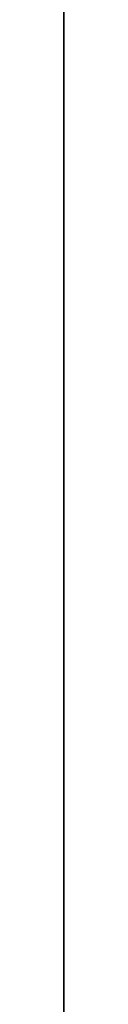
# Model space of a CAD drawing. Units: inches. Extents: x 2083 to 3317, y 1141 to 2115.
# Tile 45 of 256: x 2235.9598 to 2235.9598, y 1478.7355 to 1479.2752. Entities that reach past the tile are written whole.
import ezdxf

# ---------------------------------------------------------------- set-up
doc = ezdxf.new("R2010")
doc.units = ezdxf.units.IN
doc.layers.add('A-ANNO-DIMS', color=2, linetype='Continuous', lineweight=18)
doc.layers.add('A-WALL', color=7, linetype='Continuous', lineweight=35)
doc.layers.add('A-WALL-PATT', color=251, linetype='Continuous', lineweight=13, true_color=0x636466)
doc.styles.get("Standard").update_dxf_attribs({"font": 'arial.ttf'})
doc.dimstyles.new('ISO-25', dxfattribs={"dimtxt": 12, "dimasz": 12, "dimexe": 1.25, "dimexo": 0.625, "dimtad": 1, "dimlunit": 3, "dimtxsty": 'Standard', "dimcen": 2.5, "dimadec": 0, "dimazin": 0, "dimtfac": 1, "dimtmove": 0, "dimatfit": 3, "dimfxl": 1, "dimarcsym": 0})

# ---------------------------------------------------------------- blocks, each defined once
blk = doc.blocks.new('*D30')
at = {"layer": 'A-ANNO-DIMS', "color": 0, "lineweight": -2, "transparency": 16777216}
for p, q in [((2240.01786, 1445.27381), (2240.01786, 1448.04553)), ((2254.32933, 1445.27381), (2254.32933, 1448.04553)), ((2228.01786, 1446.79553), (2216.01786, 1446.79553)), ((2240.01786, 1446.79553), (2254.32933, 1446.79553)), ((2266.32933, 1446.79553), (2413.76487, 1446.79553))]:
    blk.add_line(p, q, dxfattribs=at)
at = {"layer": 'A-ANNO-DIMS', "color": 0, "transparency": 16777216}
for points in [[(2228.01786, 1448.79553), (2228.01786, 1444.79553), (2240.01786, 1446.79553)], [(2266.32933, 1448.79553), (2266.32933, 1444.79553), (2254.32933, 1446.79553)]]:
    blk.add_solid(points, dxfattribs=at)
at = {"layer": 'Defpoints', "color": 0, "transparency": 16777216}
for p in [(2254.32933, 1446.79553), (2240.01786, 1444.64881), (2254.32933, 1444.64881)]:
    blk.add_point(p, dxfattribs=at)
at = {"layer": 'A-ANNO-DIMS', "color": 0, "transparency": 16777216, "insert": (2346.0471, 1453.62517), "char_height": 12, "attachment_point": 5}
blk.add_mtext('WC 1\'-2 1/2" TYP.', dxfattribs=at)
blk = doc.blocks.new('*D31')
at = {"layer": 'A-ANNO-DIMS', "color": 0, "lineweight": -2, "transparency": 16777216}
for p, q in [((2237.87114, 1456.64881), (2237.87114, 1541.91518)), ((2239.39286, 1444.64881), (2236.62114, 1444.64881)), ((2237.87114, 1431.54754), (2237.87114, 1444.64881)), ((2239.39286, 1431.54754), (2236.62114, 1431.54754)), ((2237.87114, 1419.54754), (2237.87114, 1407.54754))]:
    blk.add_line(p, q, dxfattribs=at)
at = {"layer": 'A-ANNO-DIMS', "color": 0, "transparency": 16777216}
for points in [[(2235.87114, 1456.64881), (2239.87114, 1456.64881), (2237.87114, 1444.64881)], [(2235.87114, 1419.54754), (2239.87114, 1419.54754), (2237.87114, 1431.54754)]]:
    blk.add_solid(points, dxfattribs=at)
at = {"layer": 'Defpoints', "color": 0, "transparency": 16777216}
for p in [(2237.87114, 1444.64881), (2240.01786, 1444.64881), (2240.01786, 1431.54754)]:
    blk.add_point(p, dxfattribs=at)
at = {"layer": 'A-ANNO-DIMS', "color": 0, "transparency": 16777216, "insert": (2231.21749, 1505.28199), "char_height": 12, "attachment_point": 5, "rotation": 90}
blk.add_mtext('1\'-1" TYP.', dxfattribs=at)
blk = doc.blocks.new('*D45')
at = {"layer": 'A-ANNO-DIMS', "color": 0, "lineweight": -2, "transparency": 16777216}
for p, q in [((2235.95978, 1478.38636), (2235.95978, 1531.36136)), ((2418.95978, 1478.38636), (2418.95978, 1531.36136)), ((2247.95978, 1530.11136), (2406.95978, 1530.11136))]:
    blk.add_line(p, q, dxfattribs=at)
at = {"layer": 'A-ANNO-DIMS', "color": 0, "transparency": 16777216}
for points in [[(2247.95978, 1532.11136), (2247.95978, 1528.11136), (2235.95978, 1530.11136)], [(2406.95978, 1532.11136), (2406.95978, 1528.11136), (2418.95978, 1530.11136)]]:
    blk.add_solid(points, dxfattribs=at)
at = {"layer": 'Defpoints', "color": 0, "transparency": 16777216}
for p in [(2418.95978, 1530.11136), (2235.95978, 1477.76136), (2418.95978, 1477.76136)]:
    blk.add_point(p, dxfattribs=at)
at = {"layer": 'A-ANNO-DIMS', "color": 0, "transparency": 16777216, "insert": (2327.45978, 1536.86733), "char_height": 12, "attachment_point": 5}
blk.add_mtext('15\'-3"', dxfattribs=at)
blk = doc.blocks.new('*D62')
at = {"layer": 'A-ANNO-DIMS', "color": 0, "lineweight": -2, "transparency": 16777216}
for p, q in [((2235.95978, 1469.38636), (2235.95978, 1522.36136)), ((2379.95978, 1469.38636), (2379.95978, 1522.36136)), ((2247.95978, 1521.11136), (2367.95978, 1521.11136))]:
    blk.add_line(p, q, dxfattribs=at)
at = {"layer": 'A-ANNO-DIMS', "color": 0, "transparency": 16777216}
for points in [[(2247.95978, 1523.11136), (2247.95978, 1519.11136), (2235.95978, 1521.11136)], [(2367.95978, 1523.11136), (2367.95978, 1519.11136), (2379.95978, 1521.11136)]]:
    blk.add_solid(points, dxfattribs=at)
at = {"layer": 'Defpoints', "color": 0, "transparency": 16777216}
for p in [(2379.95978, 1521.11136), (2235.95978, 1468.76136), (2379.95978, 1468.76136)]:
    blk.add_point(p, dxfattribs=at)
at = {"layer": 'A-ANNO-DIMS', "color": 0, "transparency": 16777216, "insert": (2307.95978, 1527.86324), "char_height": 12, "attachment_point": 5}
blk.add_mtext('12\'-0"', dxfattribs=at)

msp = doc.modelspace()

# ---------------------------------------------------------------- hatches: boundary and pattern name
at = {"layer": 'A-WALL-PATT'}
h = msp.add_hatch(color=256, dxfattribs=at)
h.dxf.hatch_style = 1
h.paths.add_polyline_path([(3126.95978, 2020.76136), (2748.95978, 2020.76136), (2604.95978, 2020.76136), (2226.95978, 2020.76136), (2226.95978, 1702.76136), (2466.95978, 1702.76136), (2466.95978, 1582.76136), (2418.95978, 1582.76136), (2418.95978, 1477.76136), (2226.95978, 1477.76136), (2226.95978, 1263.26136), (2544.95978, 1263.26136), (2544.95978, 1411.76136), (2604.95978, 1411.76136), (2685.95978, 1411.76136), (2685.95978, 1420.76136), (2604.95978, 1420.76136), (2604.95978, 1573.76136), (2604.95978, 1702.76136), (2604.95978, 2011.76136), (2748.95978, 2011.76136), (2748.95978, 1702.76136), (2862.95978, 1702.76136), (2862.95978, 1621.76136), (2871.95978, 1621.76136), (2871.95978, 1702.76136), (2883.95978, 1702.76136), (2883.95978, 1706.93946, -0.026459), (2883.95978, 1711.76136), (2757.95978, 1711.76136), (2757.95978, 1807.76136), (2787.95978, 1807.76136), (2787.95978, 1812.26136), (2757.95978, 1812.26136), (2757.95978, 2011.76136), (2877.95978, 2011.76136), (2877.95978, 1812.26136), (2847.95978, 1812.26136), (2847.95978, 1807.76136), (2889.83574, 1807.76136), (2889.83574, 1812.26136), (2882.45978, 1812.26136), (2882.45978, 2011.76136), (3117.95978, 2011.76136), (3117.95978, 1812.26136), (2937.83574, 1812.26136), (2937.83574, 1807.76136), (2995.70978, 1807.76136), (2995.70978, 1796.11767), (3000.20978, 1796.11767), (3000.20978, 1807.76136), (3117.95978, 1807.76136), (3117.95978, 1711.76136), (3000.20978, 1711.76136), (3000.20978, 1760.11767), (2998.5727, 1760.11767, -0.020711), (2995.70978, 1760.11767), (2995.70978, 1711.76136), (2931.95978, 1711.76136), (2931.95978, 1702.76136), (3126.95978, 1702.76136)])
h.paths.add_polyline_path([(2471.45978, 2011.76136), (2471.45978, 1810.01136), (2462.71694, 1810.01136), (2462.71694, 1805.51136), (2505.95978, 1805.51136), (2505.95978, 1810.01136), (2475.95978, 1810.01136), (2475.95978, 2011.76136), (2595.95978, 2011.76136), (2595.95978, 1810.01136), (2565.95978, 1810.01136), (2565.95978, 1805.51136), (2595.95978, 1805.51136), (2595.95978, 1711.76136), (2235.95978, 1711.76136), (2235.95978, 1805.51136), (2353.70978, 1805.51136), (2353.70978, 1796.05416), (2358.20978, 1796.05416), (2358.20978, 1805.51136), (2414.71694, 1805.51136), (2414.71694, 1810.01136), (2235.95978, 1810.01136), (2235.95978, 2011.76136)], flags=16)
h.paths.add_polyline_path([(2270.20473, 1994.61001), (2270.20473, 1970.61001), (2246.20473, 1970.61001), (2246.20473, 1994.61001)], flags=0)
edge = h.paths.add_edge_path(flags=0)
edge.add_ellipse((2332.02739, 1899.79818), major_axis=(-3.04299, 3.04299), ratio=0.1682525, start_angle=-161.33217, end_angle=-156.30711, ccw=False)
edge.add_ellipse((2333.08204, 1898.74353), major_axis=(-1.05465, 1.05465), ratio=0.4535321, start_angle=-123.37102, end_angle=-94.15911)
edge = h.paths.add_edge_path(flags=0)
edge.add_ellipse((2332.02739, 1968.87629), major_axis=(3.04299, 3.04299), ratio=0.1682525, start_angle=18.66783, end_angle=23.69289)
edge.add_spline(control_points=[(2332.9256, 1970.6911), (2332.22677, 1970.3361), (2330.89371, 1969.65891), (2328.41308, 1970.93214), (2327.20393, 1967.74871), (2324.7096, 1969.95559), (2322.53282, 1967.01235), (2320.01285, 1971.29581), (2317.68031, 1968.15784), (2316.04053, 1967.10205), (2315.4269, 1966.8096)], knot_values=[0, 0, 0, 0, 2.267059, 4.324559, 6.685584, 8.878641, 11.121502, 14.300359, 17.755284, 19.732645, 19.732645, 19.732645, 19.732645], degree=3, periodic=0)
edge.add_ellipse((2332.02739, 1968.87629), major_axis=(3.04299, 3.04299), ratio=0.1682525, start_angle=18.66783, end_angle=23.69289, ccw=False)
edge.add_ellipse((2333.08204, 1969.93094), major_axis=(1.05465, 1.05465), ratio=0.4535321, start_angle=56.62898, end_angle=85.84089, ccw=False)
edge = h.paths.add_edge_path(flags=0)
edge.add_spline(control_points=[(2296.42829, 1967.98791), (2293.6278, 1965.33631), (2287.70362, 1959.72709), (2299.74386, 1949.9957), (2294.53259, 1935.66853), (2290.57323, 1920.60351), (2293.39412, 1909.97369), (2296.18541, 1904.96654)], knot_values=[0.099185, 0.099185, 0.099185, 0.099185, 0.345301, 0.619822, 0.982653, 1.386093, 1.810555, 1.810555, 1.810555, 1.810555], degree=3, periodic=0)
edge.add_spline(control_points=[(2296.18541, 1904.96654), (2297.38358, 1902.6193), (2298.00097, 1901.94931), (2298.55297, 1901.46815)], knot_values=[0.006246, 0.006246, 0.006246, 0.006246, 0.055476, 0.055476, 0.055476, 0.055476], degree=3, periodic=0)
edge.add_spline(control_points=[(2298.55297, 1901.46815), (2297.25861, 1900.92322), (2295.22529, 1900.23213), (2293.06023, 1900.61421), (2292.10142, 1900.78841), (2292.08958, 1900.79057)], knot_values=[0.312835, 0.312835, 0.312835, 0.312835, 0.40178, 0.474987, 0.475903, 0.475903, 0.475903, 0.475903], degree=3, periodic=0)
edge.add_arc((2292.79365, 1904.66411), 3.93701, 215.4209, 259.69818, ccw=False)
edge.add_spline(control_points=[(2289.58531, 1902.3823), (2289.47665, 1902.53509), (2289.36848, 1902.68804), (2289.26086, 1902.84117)], knot_values=[0.102872, 0.102872, 0.102872, 0.102872, 0.116896, 0.116896, 0.116896, 0.116896], degree=3, periodic=0)
edge.add_spline(control_points=[(2289.26086, 1902.84117), (2288.6866, 1902.55019), (2287.64005, 1902.0199), (2285.88134, 1901.87395), (2283.85297, 1901.50435), (2281.71999, 1899.71054), (2278.46699, 1899.49294), (2276.15714, 1901.8832), (2272.25895, 1899.80407), (2267.77761, 1901.84318), (2262.24388, 1900.18403), (2257.41493, 1901.78206), (2254.31837, 1900.72612), (2253.17828, 1900.33734)], knot_values=[0, 0, 0, 0, 1.907977, 3.477176, 5.261074, 7.972851, 11.680248, 13.717921, 16.939592, 22.789562, 27.502503, 33.595215, 37.145618, 37.145618, 37.145618, 37.145618], degree=3, periodic=0)
edge.add_line((2253.17828, 1900.33734), (2250.24424, 1902.84117))
edge.add_line((2250.24424, 1902.84117), (2250.24424, 1965.8333))
edge.add_line((2250.24424, 1965.8333), (2253.17828, 1968.33712))
edge.add_spline(control_points=[(2253.17828, 1968.33712), (2254.31837, 1967.94835), (2257.41493, 1966.89241), (2262.24388, 1968.49043), (2267.77761, 1966.83128), (2271.52673, 1968.53722), (2273.87591, 1967.82829), (2274.2067, 1967.72764)], knot_values=[0, 0, 0, 0, 0.09018, 0.244935, 0.364644, 0.513233, 0.537855, 0.537855, 0.537855, 0.537855], degree=3, periodic=0)
edge.add_arc((2274.35289, 1963.79335), 3.93701, 72.05113, 92.12795, ccw=False)
edge.add_arc((2281.29693, 1985.23), 18.5963, 252.051134, 288.565722)
edge.add_arc((2292.31672, 1956.02888), 12.64608, 71.026788, 113.778218, ccw=False)
edge = h.paths.add_edge_path(flags=0)
edge.add_spline(control_points=[(2274.89941, 1951.85619), (2275.06616, 1951.61659), (2275.23269, 1951.37659), (2275.39799, 1951.13585)], knot_values=[1.409916, 1.409916, 1.409916, 1.409916, 1.43159, 1.43159, 1.43159, 1.43159], degree=3, periodic=0)
edge.add_spline(control_points=[(2275.39799, 1951.13585), (2275.79211, 1950.56189), (2276.17923, 1949.98377), (2276.54555, 1949.3971)], knot_values=[1.358238, 1.358238, 1.358238, 1.358238, 1.409916, 1.409916, 1.409916, 1.409916], degree=3, periodic=0)
edge.add_line((2276.54555, 1949.3971), (2277.43729, 1947.86218))
edge.add_spline(control_points=[(2277.43729, 1947.86218), (2276.30383, 1945.67311), (2274.6397, 1942.42688), (2274.63161, 1938.0939), (2272.79912, 1930.85155), (2274.35643, 1943.89705), (2275.94768, 1947.92336), (2276.54555, 1949.3971)], knot_values=[0.005632, 0.005632, 0.005632, 0.005632, 0.186014, 0.266002, 0.357087, 0.59639, 0.739732, 0.739732, 0.739732, 0.739732], degree=3, periodic=0)
edge.add_spline(control_points=[(2276.54555, 1949.3971), (2276.17923, 1949.98377), (2275.79211, 1950.56189), (2275.39799, 1951.13585)], knot_values=[1.358238, 1.358238, 1.358238, 1.358238, 1.409916, 1.409916, 1.409916, 1.409916], degree=3, periodic=0)
edge.add_spline(control_points=[(2275.39799, 1951.13585), (2274.9425, 1950.08045), (2274.20776, 1948.02527), (2273.9346, 1944.85148), (2272.46853, 1937.62749), (2273.46622, 1945.69647), (2274.70062, 1951.05947), (2274.89941, 1951.85619)], knot_values=[0.104364, 0.104364, 0.104364, 0.104364, 0.189636, 0.269624, 0.36071, 0.600013, 0.644622, 0.644622, 0.644622, 0.644622], degree=3, periodic=0)
h.paths.add_polyline_path([(2269.16751, 1963.12757, -0.357527), (2268.17063, 1960.97637, -0.092561), (2268.17063, 1939.43632, -0.357527), (2269.16751, 1937.28512, -0.357527), (2267.01631, 1938.282, -0.164785), (2254.68558, 1938.282, -0.357527), (2252.53438, 1937.28512, -0.357527), (2253.53126, 1939.43632, -0.092561), (2253.53126, 1960.97637, -0.357527), (2252.53438, 1963.12757, -0.357527), (2254.68558, 1962.13069, -0.164785), (2267.01631, 1962.13069, -0.357527)], flags=0)
h.paths.add_polyline_path([(2248.87407, 1967.8018), (2248.87407, 1957.02771), (2249.45778, 1957.02771), (2249.45778, 1911.64676), (2248.87407, 1911.64676), (2248.87407, 1900.87267), (2246.51186, 1900.87267, 0.197327), (2244.14966, 1902.45687), (2244.14966, 1966.21759, 0.197327), (2246.51186, 1967.8018)], flags=0)
h.paths.add_polyline_path([(2269.16751, 1931.38934, -0.357527), (2268.17063, 1929.23814, -0.092561), (2268.17063, 1907.6981, -0.357527), (2269.16751, 1905.54689, -0.357527), (2267.01631, 1906.54377, -0.164785), (2254.68558, 1906.54377, -0.357527), (2252.53438, 1905.54689, -0.357527), (2253.53126, 1907.6981, -0.092561), (2253.53126, 1929.23814, -0.357527), (2252.53438, 1931.38934, -0.357527), (2254.68558, 1930.39246, -0.164785), (2267.01631, 1930.39246, -0.357527)], flags=0)
edge = h.paths.add_edge_path(flags=0)
edge.add_spline(control_points=[(2276.19686, 1906.7237), (2276.16814, 1909.02893), (2276.11405, 1913.37185), (2270.59842, 1924.92498), (2273.90517, 1919.01278), (2275.92171, 1916.26206), (2275.47457, 1912.40215), (2277.25787, 1910.38062), (2276.69604, 1908.22504), (2276.64622, 1906.81302), (2276.61782, 1906.00841)], knot_values=[0, 0, 0, 0, 8.61026, 16.221274, 18.843057, 23.804898, 27.440828, 29.356102, 31.203478, 33.650687, 33.650687, 33.650687, 33.650687], degree=3, periodic=0)
edge.add_spline(control_points=[(2276.61782, 1906.00841), (2276.62331, 1905.62414), (2276.49774, 1904.62866), (2275.44178, 1903.85473), (2274.93731, 1903.08045), (2274.85908, 1902.84117)], knot_values=[0.156488, 0.156488, 0.156488, 0.156488, 0.184398, 0.231376, 0.250598, 0.250598, 0.250598, 0.250598], degree=3, periodic=0)
edge.add_line((2274.85908, 1902.84117), (2276.50598, 1902.84117))
edge.add_spline(control_points=[(2276.50598, 1902.84117), (2276.78831, 1903.08494), (2277.66507, 1904.1252), (2278.24954, 1904.34074), (2277.65387, 1908.52739), (2278.15567, 1906.22781), (2278.10046, 1905.28595), (2278.84667, 1904.06901), (2277.85679, 1903.41495), (2277.87419, 1902.99105), (2277.90356, 1902.84117)], knot_values=[0.059574, 0.059574, 0.059574, 0.059574, 0.080753, 0.103741, 0.16972, 0.176036, 0.207137, 0.240474, 0.262341, 0.27366, 0.27366, 0.27366, 0.27366], degree=3, periodic=0)
edge.add_line((2277.90356, 1902.84117), (2280.02983, 1902.84117))
edge.add_spline(control_points=[(2280.02983, 1902.84117), (2279.88822, 1903.0884), (2279.49926, 1903.98155), (2280.15228, 1905.93935), (2278.10362, 1909.65776), (2279.76239, 1907.18529), (2280.3279, 1904.87486), (2280.48511, 1903.48959), (2281.46327, 1903.24943), (2281.75834, 1902.9365), (2281.83404, 1902.84117)], knot_values=[0.013856, 0.013856, 0.013856, 0.013856, 0.034874, 0.088867, 0.107879, 0.126738, 0.158714, 0.193757, 0.217487, 0.226722, 0.226722, 0.226722, 0.226722], degree=3, periodic=0)
edge.add_spline(control_points=[(2281.83404, 1902.84117), (2281.78753, 1902.8267), (2281.64702, 1902.78299), (2281.39553, 1902.85949), (2281.08808, 1902.98524), (2280.72068, 1903.0609), (2280.33345, 1903.02573), (2280.12477, 1902.89888), (2280.02983, 1902.84117)], knot_values=[0, 0, 0, 0, 0.14413, 0.435517, 0.749276, 1.153046, 1.548371, 1.878348, 1.878348, 1.878348, 1.878348], degree=3, periodic=0)
edge.add_line((2280.02983, 1902.84117), (2277.90356, 1902.84117))
edge.add_spline(control_points=[(2277.90356, 1902.84117), (2277.89286, 1902.79586), (2277.8654, 1902.67964), (2277.60748, 1902.68748), (2277.27405, 1902.8007), (2276.83792, 1902.61977), (2276.58381, 1902.78926), (2276.50598, 1902.84117)], knot_values=[0, 0, 0, 0, 0.127189, 0.326199, 0.628009, 1.24357, 1.515331, 1.515331, 1.515331, 1.515331], degree=3, periodic=0)
edge.add_line((2276.50598, 1902.84117), (2274.85908, 1902.84117))
edge.add_spline(control_points=[(2274.85908, 1902.84117), (2274.81444, 1902.89859), (2274.72513, 1903.01345), (2274.49348, 1903.11897), (2274.24429, 1902.96054), (2273.93712, 1903.18494), (2273.61404, 1902.98314), (2273.40832, 1902.88304), (2273.32225, 1902.84117)], knot_values=[0, 0, 0, 0, 0.21843, 0.436957, 0.687977, 0.990379, 1.398396, 1.69185, 1.69185, 1.69185, 1.69185], degree=3, periodic=0)
edge.add_spline(control_points=[(2273.32225, 1902.84117), (2273.61674, 1903.44569), (2274.274, 1904.53825), (2276.02724, 1904.5737), (2276.20696, 1906.58364), (2276.19686, 1906.7237)], knot_values=[0.012227, 0.012227, 0.012227, 0.012227, 0.059472, 0.106218, 0.134458, 0.134458, 0.134458, 0.134458], degree=3, periodic=0)
h.paths.add_polyline_path([(2270.77605, 1897.78983), (2270.77605, 1873.78983), (2246.77605, 1873.78983), (2246.77605, 1897.78983)], flags=0)
h.paths.add_polyline_path([(2353.70978, 1760.00506), (2353.70978, 1760.05416), (2358.20978, 1760.05416, -0.033729)], flags=0)
h.paths.add_polyline_path([(2321.81912, 1737.52919), (2341.99533, 1737.52919, -0.414214), (2343.20327, 1736.32124), (2343.20327, 1721.0206, -0.414214), (2341.99533, 1719.81265), (2321.81912, 1719.81265, -0.414214), (2320.61117, 1721.0206), (2320.61117, 1736.32124, -0.414214)], flags=0)
h.paths.add_polyline_path([(2324.23501, 1736.32124), (2339.57944, 1736.32124, -0.414214), (2341.99533, 1733.90535), (2341.99533, 1725.44973, -0.414214), (2339.57944, 1723.03384), (2333.68059, 1723.03384), (2333.84532, 1722.04547, -0.870646), (2335.4254, 1721.82589, -0.767327), (2333.92269, 1721.42324), (2331.29102, 1721.42324, -0.767327), (2329.78832, 1721.82589, -0.870646), (2331.3684, 1722.04547), (2331.53313, 1723.03384), (2324.23501, 1723.03384, -0.414214), (2321.81912, 1725.44973), (2321.81912, 1733.90535, -0.414214)], flags=0)
h.paths.add_polyline_path([(2570.48379, 1928.61544), (2589.68379, 1928.61544), (2590.16883, 1928.61544), (2590.16883, 1904.9934), (2570.48379, 1904.9934)], flags=0)
h.paths.add_polyline_path([(2574.44732, 1927.26382, -1), (2572.82884, 1927.26382, -1)], flags=0)
h.paths.add_polyline_path([(2573.08987, 1926.94088), (2573.92503, 1927.77604), (2574.14774, 1927.55333), (2573.31258, 1926.71817)], flags=0)
h.paths.add_polyline_path([(2578.77906, 1919.72962, -1), (2571.59166, 1919.72962, -1)], flags=0)
h.paths.add_polyline_path([(2578.38536, 1919.72962, -1), (2571.98536, 1919.72962, -1)], flags=0)
h.paths.add_polyline_path([(2331.59576, 1729.47622, -1), (2333.61795, 1729.47622, -1)], flags=0)
h.paths.add_polyline_path([(2578.03423, 1927.26382, -1), (2576.41574, 1927.26382, -1)], flags=0)
h.paths.add_polyline_path([(2576.68885, 1927.53109), (2576.91156, 1927.7538), (2577.74673, 1926.91863), (2577.52402, 1926.69592)], flags=0)
h.paths.add_polyline_path([(2578.13906, 1909.85954, -1), (2572.23166, 1909.85954, -1)], flags=0)
h.paths.add_polyline_path([(2577.74536, 1909.85954, -1), (2572.62536, 1909.85954, -1)], flags=0)
h.paths.add_polyline_path([(2583.79772, 1927.26382, -1), (2582.17923, 1927.26382, -1)], flags=0)
h.paths.add_polyline_path([(2582.71865, 1927.7538), (2583.55381, 1926.91863), (2583.3311, 1926.69592), (2582.49594, 1927.53109)], flags=0)
h.paths.add_polyline_path([(2582.49594, 1927.53109), (2582.71865, 1927.7538), (2583.55381, 1926.91863), (2583.3311, 1926.69592)], flags=0)
h.paths.add_polyline_path([(2587.73906, 1920.52962, -1), (2581.83166, 1920.52962, -1)], flags=0)
h.paths.add_polyline_path([(2587.34536, 1920.52962, -1), (2582.22536, 1920.52962, -1)], flags=0)
h.paths.add_polyline_path([(2587.38462, 1927.26382, -1), (2585.76613, 1927.26382, -1)], flags=0)
h.paths.add_polyline_path([(2586.08199, 1926.98025), (2586.91716, 1927.81541), (2587.13987, 1927.5927), (2586.3047, 1926.75754)], flags=0)
h.paths.add_polyline_path([(2588.37906, 1910.65954, -1), (2581.19166, 1910.65954, -1)], flags=0)
h.paths.add_polyline_path([(2587.98536, 1910.65954, -1), (2581.58536, 1910.65954, -1)], flags=0)
h.paths.add_polyline_path([(2417.16773, 1729.4779), (2437.34394, 1729.4779, -0.414214), (2438.55188, 1728.26995), (2438.55188, 1712.96931, -0.414214), (2437.34394, 1711.76136), (2417.16773, 1711.76136, -0.414214), (2415.95978, 1712.96931), (2415.95978, 1728.26995, -0.414214)], flags=0)
h.paths.add_polyline_path([(2419.58362, 1728.26995), (2434.92805, 1728.26995, -0.414214), (2437.34394, 1725.85406), (2437.34394, 1717.39844, -0.414214), (2434.92805, 1714.98255), (2429.0292, 1714.98255), (2429.19393, 1713.99418, -0.870646), (2430.77401, 1713.7746, -0.767327), (2429.2713, 1713.37195), (2426.63963, 1713.37195, -0.767327), (2425.13693, 1713.7746, -0.870646), (2426.71701, 1713.99418), (2426.88174, 1714.98255), (2419.58362, 1714.98255, -0.414214), (2417.16773, 1717.39844), (2417.16773, 1725.85406, -0.414214)], flags=0)
h.paths.add_polyline_path([(2419.58362, 1728.26995), (2434.92805, 1728.26995, -0.414214), (2437.34394, 1725.85406), (2437.34394, 1717.39844, -0.414214), (2434.92805, 1714.98255), (2429.0292, 1714.98255), (2428.35812, 1719.00903), (2427.55282, 1719.00903), (2426.88174, 1714.98255), (2419.58362, 1714.98255, -0.414214), (2417.16773, 1717.39844), (2417.16773, 1725.85406, -0.414214)], flags=0)
h.paths.add_polyline_path([(2426.94437, 1721.42492, -1), (2428.96656, 1721.42492, -1)], flags=0)
h.paths.add_polyline_path([(2475.95978, 1702.76136), (2595.95978, 1702.76136), (2595.95978, 1582.76136), (2475.95978, 1582.76136)], flags=16)
h.paths.add_polyline_path([(2427.95978, 1573.76136), (2595.95978, 1573.76136), (2595.95978, 1468.76136), (2595.95978, 1420.76136), (2384.45978, 1420.76136), (2384.45978, 1468.76136), (2427.95978, 1468.76136)], flags=16)
h.paths.add_polyline_path([(2379.95978, 1468.76136), (2379.95978, 1420.76136), (2235.95978, 1420.76136), (2235.95978, 1468.76136)], flags=16)
h.paths.add_polyline_path([(2317.816, 1466.69577), (2337.9922, 1466.69577, -0.414214), (2339.20015, 1465.48782), (2339.20015, 1450.18718, -0.414214), (2337.9922, 1448.97923), (2317.816, 1448.97923, -0.414214), (2316.60805, 1450.18718), (2316.60805, 1465.48782, -0.414214)], flags=0)
h.paths.add_polyline_path([(2320.23189, 1465.48782), (2335.57631, 1465.48782, -0.414214), (2337.9922, 1463.07193), (2337.9922, 1454.61631, -0.414214), (2335.57631, 1452.20042), (2329.67747, 1452.20042), (2329.84219, 1451.21205, -0.870646), (2331.42228, 1450.99247, -0.767327), (2329.91957, 1450.58983), (2327.2879, 1450.58983, -0.767327), (2325.7852, 1450.99247, -0.870646), (2327.36528, 1451.21205), (2327.53001, 1452.20042), (2320.23189, 1452.20042, -0.414214), (2317.816, 1454.61631), (2317.816, 1463.07193, -0.414214)], flags=0)
h.paths.add_polyline_path([(2320.23189, 1465.48782), (2335.57631, 1465.48782, -0.414214), (2337.9922, 1463.07193), (2337.9922, 1454.61631, -0.414214), (2335.57631, 1452.20042), (2329.67747, 1452.20042), (2329.00638, 1456.22691), (2328.20109, 1456.22691), (2327.53001, 1452.20042), (2320.23189, 1452.20042, -0.414214), (2317.816, 1454.61631), (2317.816, 1463.07193, -0.414214)], flags=0)
h.paths.add_polyline_path([(2327.59264, 1458.6428, -1), (2329.61483, 1458.6428, -1)], flags=0)
h.paths.add_polyline_path([(2244.41174, 1433.34045), (2241.92094, 1433.34045, -0.414214), (2240.01786, 1435.24354), (2240.01786, 1440.95281, -0.414211), (2241.92093, 1442.8559), (2244.41174, 1442.8559, -1.976472)], flags=0)
h.paths.add_polyline_path([(2245.35689, 1434.39754, -0.414214), (2245.35689, 1441.79881, -2.144098)], flags=0)
h.paths.add_polyline_path([(2535.95978, 1416.26136), (2535.95978, 1272.26136), (2235.95978, 1272.26136), (2235.95978, 1416.26136)], flags=16)
h.paths.add_polyline_path([(2260.11956, 1384.29284), (2260.11956, 1362.03865), (2237.86537, 1362.03865), (2237.86537, 1384.29284)], flags=0)
edge = h.paths.add_edge_path(flags=0)
edge.add_line((2318.25185, 1362.0933), (2318.1458, 1362.00097))
edge.add_ellipse((2317.44512, 1360.43104), major_axis=(2.82164, 2.82164), ratio=0.1682525, start_angle=18.66783, end_angle=20.94813, ccw=False)
edge.add_ellipse((2318.42305, 1361.40897), major_axis=(0.97793, 0.97793), ratio=0.4535321, start_angle=56.62898, end_angle=70.2262, ccw=False)
edge = h.paths.add_edge_path(flags=0)
edge.add_line((2319.10737, 1295.57108), (2319.01504, 1295.67713))
edge.add_ellipse((2317.44512, 1296.37781), major_axis=(-2.82164, 2.82164), ratio=0.1682525, start_angle=-161.33217, end_angle=-159.05187, ccw=False)
edge.add_ellipse((2318.42305, 1295.39988), major_axis=(-0.97793, 0.97793), ratio=0.4535321, start_angle=-123.37102, end_angle=-109.7738)
edge = h.paths.add_edge_path(flags=0)
edge.add_spline(control_points=[(2284.21035, 1301.17022), (2284.58069, 1300.44472), (2284.89119, 1299.89202), (2285.15955, 1299.46102)], knot_values=[0.039066, 0.039066, 0.039066, 0.039066, 0.055476, 0.055476, 0.055476, 0.055476], degree=3, periodic=0)
edge.add_line((2285.15955, 1299.46102), (2284.21035, 1301.17022))
edge = h.paths.add_edge_path(flags=0)
edge.add_line((2280.41246, 1297.29801), (2283.36999, 1297.03612))
edge.add_line((2283.36999, 1297.03612), (2286.40569, 1297.92631))
edge.add_spline(control_points=[(2286.40569, 1297.92631), (2285.30549, 1297.46312), (2284.34478, 1297.12915), (2283.36999, 1297.03612)], knot_values=[0.394369, 0.394369, 0.394369, 0.394369, 0.475903, 0.475903, 0.475903, 0.475903], degree=3, periodic=0)
edge.add_spline(control_points=[(2283.36999, 1297.03612), (2283.28139, 1297.02767), (2282.31629, 1296.95734), (2281.3125, 1297.13448), (2280.42344, 1297.29602), (2280.41246, 1297.29801)], knot_values=[0.312835, 0.312835, 0.312835, 0.312835, 0.320246, 0.393453, 0.394369, 0.394369, 0.394369, 0.394369], degree=3, periodic=0)
edge = h.paths.add_edge_path(flags=0)
edge.add_line((2284.43556, 1359.60729), (2280.44629, 1355.32805))
edge.add_line((2280.44629, 1355.32805), (2279.57999, 1351.01775))
edge.add_line((2279.57999, 1351.01775), (2282.41297, 1346.58043))
edge.add_spline(control_points=[(2282.41297, 1346.58043), (2283.15333, 1345.58924), (2284.2529, 1344.0289), (2284.80104, 1342.38717), (2284.93516, 1341.80554)], knot_values=[1.240098, 1.240098, 1.240098, 1.240098, 1.332892, 1.382712, 1.382712, 1.382712, 1.382712], degree=3, periodic=0)
edge.add_spline(control_points=[(2284.93516, 1341.80554), (2285.31911, 1340.1406), (2285.23303, 1338.4092), (2284.90994, 1336.65412)], knot_values=[1.097484, 1.097484, 1.097484, 1.097484, 1.240098, 1.240098, 1.240098, 1.240098], degree=3, periodic=0)
edge.add_spline(control_points=[(2284.90994, 1336.65412), (2284.58685, 1334.89904), (2284.02675, 1333.12027), (2283.46264, 1331.36058)], knot_values=[0.95487, 0.95487, 0.95487, 0.95487, 1.097484, 1.097484, 1.097484, 1.097484], degree=3, periodic=0)
edge.add_line((2283.46264, 1331.36058), (2281.89038, 1326.15336))
edge.add_line((2281.89038, 1326.15336), (2280.75626, 1321.05609))
edge.add_line((2280.75626, 1321.05609), (2280.2992, 1316.00198))
edge.add_line((2280.2992, 1316.00198), (2280.71593, 1310.95007))
edge.add_line((2280.71593, 1310.95007), (2282.02809, 1305.97214))
edge.add_line((2282.02809, 1305.97214), (2284.21035, 1301.17022))
edge.add_spline(control_points=[(2284.21035, 1301.17022), (2283.34073, 1302.73019), (2282.6119, 1304.33649), (2282.02809, 1305.97214)], knot_values=[0.099185, 0.099185, 0.099185, 0.099185, 0.241799, 0.241799, 0.241799, 0.241799], degree=3, periodic=0)
edge.add_spline(control_points=[(2282.02809, 1305.97214), (2281.44428, 1307.60778), (2281.00549, 1309.27276), (2280.71593, 1310.95007)], knot_values=[0.241799, 0.241799, 0.241799, 0.241799, 0.384413, 0.384413, 0.384413, 0.384413], degree=3, periodic=0)
edge.add_spline(control_points=[(2280.71593, 1310.95007), (2280.43324, 1312.58761), (2280.28939, 1314.27696), (2280.29889, 1315.96203), (2280.2992, 1316.00198)], knot_values=[0.384413, 0.384413, 0.384413, 0.384413, 0.523647, 0.527028, 0.527028, 0.527028, 0.527028], degree=3, periodic=0)
edge.add_spline(control_points=[(2280.2992, 1316.00198), (2280.31233, 1317.68696), (2280.47787, 1319.36793), (2280.75626, 1321.05609)], knot_values=[0.527028, 0.527028, 0.527028, 0.527028, 0.669642, 0.669642, 0.669642, 0.669642], degree=3, periodic=0)
edge.add_spline(control_points=[(2280.75626, 1321.05609), (2281.03465, 1322.74425), (2281.42588, 1324.43961), (2281.89038, 1326.15336)], knot_values=[0.669642, 0.669642, 0.669642, 0.669642, 0.812256, 0.812256, 0.812256, 0.812256], degree=3, periodic=0)
edge.add_spline(control_points=[(2281.89038, 1326.15336), (2282.26438, 1327.53325), (2282.78787, 1329.26181), (2283.35275, 1331.01778), (2283.46264, 1331.36058)], knot_values=[0.812256, 0.812256, 0.812256, 0.812256, 0.927087, 0.95487, 0.95487, 0.95487, 0.95487], degree=3, periodic=0)
edge.add_line((2283.46264, 1331.36058), (2284.90994, 1336.65412))
edge.add_line((2284.90994, 1336.65412), (2284.93516, 1341.80554))
edge.add_line((2284.93516, 1341.80554), (2282.41297, 1346.58043))
edge.add_spline(control_points=[(2282.41297, 1346.58043), (2281.27513, 1348.10379), (2280.07845, 1349.57032), (2279.57999, 1351.01775)], knot_values=[1.382712, 1.382712, 1.382712, 1.382712, 1.525326, 1.525326, 1.525326, 1.525326], degree=3, periodic=0)
edge.add_spline(control_points=[(2279.57999, 1351.01775), (2279.44328, 1351.41472), (2279.13631, 1352.85692), (2279.73519, 1354.29039), (2280.44629, 1355.32805)], knot_values=[1.525326, 1.525326, 1.525326, 1.525326, 1.564439, 1.667941, 1.667941, 1.667941, 1.667941], degree=3, periodic=0)
edge.add_spline(control_points=[(2280.44629, 1355.32805), (2281.42611, 1356.75784), (2282.93084, 1358.18256), (2284.43556, 1359.60729)], knot_values=[1.667941, 1.667941, 1.667941, 1.667941, 1.810555, 1.810555, 1.810555, 1.810555], degree=3, periodic=0)
edge.add_arc((2280.62307, 1348.51818), 11.72618, 71.026788, 113.778218)
edge.add_arc((2270.40489, 1375.59516), 17.24357, 252.051134, 288.565722, ccw=False)
edge.add_arc((2263.96597, 1355.71785), 3.65062, 72.05113, 92.12795)
edge.add_arc((2263.96597, 1355.71785), 3.65062, 92.12795, 177.98513)
edge.add_spline(control_points=[(2260.3176, 1355.8462), (2260.26042, 1354.22067), (2260.55128, 1350.18655), (2262.99934, 1346.76625), (2264.47274, 1344.64902)], knot_values=[1.43159, 1.43159, 1.43159, 1.43159, 1.564144, 1.770695, 1.770695, 1.770695, 1.770695], degree=3, periodic=0)
edge.add_line((2264.47274, 1344.64902), (2264.93559, 1343.98253))
edge.add_spline(control_points=[(2263.80104, 1340.24811), (2263.84324, 1340.51409), (2264.06724, 1341.75647), (2264.51269, 1343.00245), (2264.93505, 1343.98108)], knot_values=[0.53657, 0.53657, 0.53657, 0.53657, 0.559349, 0.644622, 0.644622, 0.644622, 0.644622], degree=3, periodic=0)
edge.add_spline(control_points=[(2264.93505, 1343.98108), (2265.11777, 1343.71497), (2265.29888, 1343.44791), (2265.47676, 1343.17936)], knot_values=[1.384077, 1.384077, 1.384077, 1.384077, 1.409916, 1.409916, 1.409916, 1.409916], degree=3, periodic=0)
edge.add_spline(control_points=[(2265.47676, 1343.17936), (2265.65464, 1342.91082), (2265.8293, 1342.64081), (2265.99913, 1342.36881)], knot_values=[1.358238, 1.358238, 1.358238, 1.358238, 1.384077, 1.384077, 1.384077, 1.384077], degree=3, periodic=0)
edge.add_line((2265.99913, 1342.36881), (2266.82601, 1340.94555))
edge.add_spline(control_points=[(2266.82601, 1340.94555), (2268.8944, 1337.08969), (2271.39817, 1325.843), (2270.51616, 1310.56856), (2275.91938, 1301.86061), (2277.78951, 1299.19945)], knot_values=[0.116896, 0.116896, 0.116896, 0.116896, 0.472987, 1.050969, 1.313793, 1.313793, 1.313793, 1.313793], degree=3, periodic=0)
edge.add_spline(control_points=[(2277.78951, 1299.19945), (2277.83941, 1299.12845), (2277.88943, 1299.0575), (2277.93957, 1298.98658)], knot_values=[0.109884, 0.109884, 0.109884, 0.109884, 0.116896, 0.116896, 0.116896, 0.116896], degree=3, periodic=0)
edge.add_line((2277.93957, 1298.98658), (2277.78885, 1299.19911))
edge.add_spline(control_points=[(2277.78885, 1299.19911), (2277.25658, 1298.92941), (2276.28635, 1298.4379), (2275.03935, 1298.33442), (2274.38333, 1298.2389), (2274.21525, 1298.20934)], knot_values=[33.12187, 33.12187, 33.12187, 33.12187, 35.029056, 36.598255, 37.144827, 37.144827, 37.144827, 37.144827], degree=3, periodic=0)
edge.add_line((2274.21525, 1298.20934), (2273.07315, 1297.89296))
edge.add_spline(control_points=[(2273.07315, 1297.89296), (2272.32294, 1297.57978), (2271.03915, 1296.51051), (2269.24839, 1296.22606), (2268.4231, 1296.37465)], knot_values=[26.532584, 26.532584, 26.532584, 26.532584, 29.198919, 31.839101, 31.839101, 31.839101, 31.839101], degree=3, periodic=0)
edge.add_line((2268.4231, 1296.37465), (2263.8785, 1297.45753))
edge.add_spline(control_points=[(2263.8785, 1297.45753), (2263.55608, 1297.35943), (2261.86031, 1296.83869), (2260.23878, 1297.28241), (2258.93345, 1297.51646)], knot_values=[15.919551, 15.919551, 15.919551, 15.919551, 16.939592, 21.226067, 21.226067, 21.226067, 21.226067], degree=3, periodic=0)
edge.add_line((2258.93345, 1297.51646), (2254.05523, 1297.32901))
edge.add_spline(control_points=[(2254.05523, 1297.32901), (2253.75553, 1297.29582), (2252.11368, 1297.16517), (2250.46187, 1297.54422), (2249.12969, 1297.66788)], knot_values=[5.306517, 5.306517, 5.306517, 5.306517, 6.276435, 10.613034, 10.613034, 10.613034, 10.613034], degree=3, periodic=0)
edge.add_line((2249.12969, 1297.66788), (2244.33165, 1296.87776))
edge.add_line((2244.33165, 1296.87776), (2241.61103, 1299.19945))
edge.add_line((2241.61103, 1299.19945), (2241.61103, 1357.6094))
edge.add_line((2241.61103, 1357.6094), (2244.33165, 1359.9311))
edge.add_line((2244.33165, 1359.9311), (2252.72882, 1359.54269))
edge.add_spline(control_points=[(2252.72882, 1359.54269), (2252.87094, 1359.54644), (2253.30574, 1359.54817), (2253.73984, 1359.51427), (2254.03174, 1359.48243)], knot_values=[0.233291, 0.233291, 0.233291, 0.233291, 0.244935, 0.268927, 0.268927, 0.268927, 0.268927], degree=3, periodic=0)
edge.add_line((2254.03174, 1359.48243), (2259.58719, 1359.41639))
edge.add_spline(control_points=[(2259.58719, 1359.41639), (2260.67707, 1359.6285), (2262.0732, 1359.897), (2263.52369, 1359.45928), (2263.83042, 1359.36595)], knot_values=[0.422516, 0.422516, 0.422516, 0.422516, 0.513233, 0.537855, 0.537855, 0.537855, 0.537855], degree=3, periodic=0)
edge.add_arc((2263.96597, 1355.71785), 3.65062, 72.05113, 92.12795, ccw=False)
edge.add_arc((2270.40489, 1375.59516), 17.24357, 252.051134, 288.565722)
edge.add_arc((2280.62307, 1348.51818), 11.72618, 71.026788, 113.778218, ccw=False)
h.paths.add_polyline_path([(2240.34053, 1359.43471), (2240.34053, 1349.44435), (2240.88178, 1349.44435), (2240.88178, 1307.3645), (2240.34053, 1307.3645), (2240.34053, 1297.37414), (2238.15016, 1297.37414, 0.197327), (2235.95978, 1298.84311), (2235.95978, 1357.96575, 0.197327), (2238.15016, 1359.43471)], flags=0)
h.paths.add_polyline_path([(2259.15779, 1355.1005, -0.357527), (2258.23342, 1353.10578, -0.092561), (2258.23342, 1333.1326, -0.357527), (2259.15779, 1331.13788, -0.357527), (2257.16307, 1332.06225, -0.164785), (2245.7293, 1332.06225, -0.357527), (2243.73458, 1331.13788, -0.357527), (2244.65895, 1333.1326, -0.092561), (2244.65895, 1353.10578, -0.357527), (2243.73458, 1355.1005, -0.357527), (2245.7293, 1354.17613, -0.164785), (2257.16307, 1354.17613, -0.357527)], flags=0)
edge = h.paths.add_edge_path(flags=0)
edge.add_line((2265.99913, 1342.36881), (2266.82601, 1340.94555))
edge.add_line((2266.82601, 1340.94555), (2265.30756, 1337.81407))
edge.add_line((2265.30756, 1337.81407), (2264.35823, 1334.65294))
edge.add_line((2264.35823, 1334.65294), (2264.26201, 1333.7997))
edge.add_spline(control_points=[(2264.26201, 1333.7997), (2264.20836, 1333.18705), (2264.16206, 1332.36553), (2264.00714, 1331.41393), (2263.96905, 1331.20183)], knot_values=[0.464444, 0.464444, 0.464444, 0.464444, 0.516691, 0.531608, 0.531608, 0.531608, 0.531608], degree=3, periodic=0)
edge.add_spline(control_points=[(2263.96905, 1331.20183), (2263.77453, 1330.11887), (2263.42437, 1328.79084), (2263.25742, 1328.53065), (2263.23403, 1328.51461)], knot_values=[0.372682, 0.372682, 0.372682, 0.372682, 0.44885, 0.464444, 0.464444, 0.464444, 0.464444], degree=3, periodic=0)
edge.add_spline(control_points=[(2263.23403, 1328.51461), (2263.09638, 1328.42023), (2263.13117, 1329.30148), (2263.27495, 1330.61575)], knot_values=[0.280919, 0.280919, 0.280919, 0.280919, 0.372682, 0.372682, 0.372682, 0.372682], degree=3, periodic=0)
edge.add_spline(control_points=[(2263.27495, 1330.61575), (2263.41874, 1331.93002), (2263.67152, 1333.67732), (2263.96985, 1335.31503)], knot_values=[0.189157, 0.189157, 0.189157, 0.189157, 0.280919, 0.280919, 0.280919, 0.280919], degree=3, periodic=0)
edge.add_spline(control_points=[(2263.96985, 1335.31503), (2264.1005, 1336.03219), (2264.41878, 1337.62191), (2264.75485, 1338.86443), (2264.94742, 1339.49112)], knot_values=[0.097394, 0.097394, 0.097394, 0.097394, 0.137578, 0.189157, 0.189157, 0.189157, 0.189157], degree=3, periodic=0)
edge.add_spline(control_points=[(2264.94742, 1339.49112), (2265.29002, 1340.60605), (2265.64424, 1341.494), (2265.99913, 1342.36881)], knot_values=[0.005632, 0.005632, 0.005632, 0.005632, 0.097394, 0.097394, 0.097394, 0.097394], degree=3, periodic=0)
h.paths.add_polyline_path([(2259.15779, 1325.67097, -0.357527), (2258.23342, 1323.67625, -0.092561), (2258.23342, 1303.70307, -0.357527), (2259.15779, 1301.70835, -0.357527), (2257.16307, 1302.63272, -0.164785), (2245.7293, 1302.63272, -0.357527), (2243.73458, 1301.70835, -0.357527), (2244.65895, 1303.70307, -0.092561), (2244.65895, 1323.67625, -0.357527), (2243.73458, 1325.67097, -0.357527), (2245.7293, 1324.74661, -0.164785), (2257.16307, 1324.74661, -0.357527)], flags=0)
edge = h.paths.add_edge_path(flags=0)
edge.add_spline(control_points=[(2261.70894, 1317.31142), (2261.67948, 1317.41758), (2261.76186, 1317.38853), (2262.49074, 1316.08987), (2262.96218, 1315.3009)], knot_values=[14.955861, 14.955861, 14.955861, 14.955861, 16.221274, 18.694826, 18.694826, 18.694826, 18.694826], degree=3, periodic=0)
edge.add_spline(control_points=[(2262.96218, 1315.3009), (2262.99044, 1315.25362), (2263.7021, 1314.06738), (2264.34898, 1313.12715), (2264.73005, 1312.16415)], knot_values=[18.694826, 18.694826, 18.694826, 18.694826, 18.843057, 22.433791, 22.433791, 22.433791, 22.433791], degree=3, periodic=0)
edge.add_spline(control_points=[(2264.73005, 1312.16415), (2264.87556, 1311.79644), (2265.17687, 1310.76981), (2265.14307, 1309.55926), (2265.24774, 1308.82419)], knot_values=[22.433791, 22.433791, 22.433791, 22.433791, 23.804898, 26.172756, 26.172756, 26.172756, 26.172756], degree=3, periodic=0)
edge.add_line((2265.24774, 1308.82419), (2265.85077, 1307.17189))
edge.add_spline(control_points=[(2265.85077, 1307.17189), (2266.06502, 1306.82168), (2266.38439, 1306.33225), (2266.4244, 1305.78055), (2266.42037, 1305.61122)], knot_values=[28.062562, 28.062562, 28.062562, 28.062562, 29.356102, 29.911721, 29.911721, 29.911721, 29.911721], degree=3, periodic=0)
edge.add_spline(control_points=[(2266.42037, 1305.61122), (2266.41612, 1305.43259), (2266.394, 1305.25), (2266.36478, 1305.06586)], knot_values=[29.911721, 29.911721, 29.911721, 29.911721, 30.497837, 30.497837, 30.497837, 30.497837], degree=3, periodic=0)
edge.add_line((2266.36478, 1305.06586), (2266.06615, 1302.1363))
edge.add_spline(control_points=[(2266.06615, 1302.1363), (2266.07124, 1301.77998), (2265.99808, 1301.19998), (2265.66327, 1300.75896), (2265.50891, 1300.58588)], knot_values=[0.156488, 0.156488, 0.156488, 0.156488, 0.184398, 0.203543, 0.203543, 0.203543, 0.203543], degree=3, periodic=0)
edge.add_line((2265.50891, 1300.58588), (2264.43534, 1299.19945))
edge.add_line((2264.43534, 1299.19945), (2265.96244, 1299.19945))
edge.add_line((2265.96244, 1299.19945), (2267.33599, 1301.17528))
edge.add_line((2267.33599, 1301.17528), (2267.31167, 1301.98624))
edge.add_spline(control_points=[(2267.31167, 1301.98624), (2267.26111, 1302.8624), (2267.16021, 1303.73713), (2267.27149, 1303.3259)], knot_values=[0.126229, 0.126229, 0.126229, 0.126229, 0.166617, 0.166617, 0.166617, 0.166617], degree=3, periodic=0)
edge.add_spline(control_points=[(2267.27149, 1303.3259), (2267.28003, 1303.2943), (2267.30979, 1303.17537), (2267.37345, 1302.88361), (2267.40612, 1302.68283), (2267.41793, 1302.60103)], knot_values=[0.166617, 0.166617, 0.166617, 0.166617, 0.16972, 0.176036, 0.180765, 0.180765, 0.180765, 0.180765], degree=3, periodic=0)
edge.add_spline(control_points=[(2267.74389, 1300.9875), (2267.68758, 1301.15094), (2267.48052, 1301.65666), (2267.48375, 1302.14479), (2267.41793, 1302.60103)], knot_values=[0.180765, 0.180765, 0.180765, 0.180765, 0.193767, 0.220139, 0.220139, 0.220139, 0.220139], degree=3, periodic=0)
edge.add_line((2267.41793, 1302.60103), (2267.74389, 1300.9875))
edge.add_spline(control_points=[(2267.74389, 1300.9875), (2267.83196, 1300.73188), (2267.93202, 1300.3099), (2267.55484, 1299.97452), (2267.42937, 1299.82921)], knot_values=[0.220139, 0.220139, 0.220139, 0.220139, 0.240474, 0.25489, 0.25489, 0.25489, 0.25489], degree=3, periodic=0)
edge.add_line((2267.42937, 1299.82921), (2267.25836, 1299.19945))
edge.add_line((2267.25836, 1299.19945), (2269.22996, 1299.19945))
edge.add_spline(control_points=[(2269.22996, 1299.19945), (2269.09865, 1299.42869), (2268.84277, 1300.01625), (2269.01157, 1300.91592), (2268.9468, 1301.66074)], knot_values=[0.013856, 0.013856, 0.013856, 0.013856, 0.034874, 0.067073, 0.067073, 0.067073, 0.067073], degree=3, periodic=0)
edge.add_line((2268.9468, 1301.66074), (2268.43158, 1303.60311))
edge.add_spline(control_points=[(2268.43158, 1303.60311), (2268.1756, 1304.19237), (2267.59621, 1305.2513), (2268.0407, 1304.62321), (2268.25139, 1304.28242)], knot_values=[0.090155, 0.090155, 0.090155, 0.090155, 0.107879, 0.120289, 0.120289, 0.120289, 0.120289], degree=3, periodic=0)
edge.add_spline(control_points=[(2268.25139, 1304.28242), (2268.36088, 1304.10533), (2269.05775, 1302.91798), (2269.38269, 1301.59042), (2269.52141, 1300.77593), (2269.57522, 1300.55578)], knot_values=[0.120289, 0.120289, 0.120289, 0.120289, 0.126738, 0.158714, 0.173506, 0.173506, 0.173506, 0.173506], degree=3, periodic=0)
edge.add_line((2269.57522, 1300.55578), (2270.6858, 1299.42126))
edge.add_spline(control_points=[(2270.6858, 1299.42126), (2270.76722, 1299.35725), (2270.83785, 1299.2814), (2270.90292, 1299.19945)], knot_values=[0.21816, 0.21816, 0.21816, 0.21816, 0.226722, 0.226722, 0.226722, 0.226722], degree=3, periodic=0)
edge.add_line((2270.9372, 1299.19291), (2270.90292, 1299.19945))
edge.add_spline(control_points=[(2270.90292, 1299.19945), (2270.85981, 1299.18603), (2270.72951, 1299.1455), (2270.49631, 1299.21644), (2270.27166, 1299.30832), (2270.12102, 1299.34796), (2270.06334, 1299.35956)], knot_values=[0.939174, 0.939174, 0.939174, 0.939174, 1.083304, 1.374691, 1.68845, 1.878348, 1.878348, 1.878348, 1.878348], degree=3, periodic=0)
edge.add_line((2270.06334, 1299.35956), (2269.22996, 1299.19945))
edge.add_line((2269.22996, 1299.19945), (2267.25836, 1299.19945))
edge.add_spline(control_points=[(2267.25836, 1299.19945), (2267.24843, 1299.15743), (2267.22297, 1299.04967), (2266.98382, 1299.05694), (2266.80921, 1299.11623), (2266.6769, 1299.10909), (2266.63653, 1299.10481)], knot_values=[0.757665, 0.757665, 0.757665, 0.757665, 0.884854, 1.083864, 1.385675, 1.515331, 1.515331, 1.515331, 1.515331], degree=3, periodic=0)
edge.add_spline(control_points=[(2266.63653, 1299.10481), (2266.48522, 1299.08879), (2266.23581, 1299.01712), (2266.03461, 1299.15132), (2265.96244, 1299.19945)], knot_values=[0, 0, 0, 0, 0.485905, 0.757665, 0.757665, 0.757665, 0.757665], degree=3, periodic=0)
edge.add_line((2265.96244, 1299.19945), (2264.43534, 1299.19945))
edge.add_line((2264.43534, 1299.19945), (2263.85844, 1299.36712))
edge.add_spline(control_points=[(2263.85844, 1299.36712), (2263.81894, 1299.37091), (2263.77953, 1299.38572), (2263.74013, 1299.4015)], knot_values=[0.845925, 0.845925, 0.845925, 0.845925, 0.978627, 0.978627, 0.978627, 0.978627], degree=3, periodic=0)
edge.add_line((2263.72179, 1299.39643), (2263.01031, 1299.19945))
edge.add_spline(control_points=[(2263.01031, 1299.19945), (2263.24579, 1299.68286), (2263.50603, 1300.12811), (2263.87349, 1300.40803)], knot_values=[0.012227, 0.012227, 0.012227, 0.012227, 0.052971, 0.052971, 0.052971, 0.052971], degree=3, periodic=0)
edge.add_spline(control_points=[(2263.87349, 1300.40803), (2263.93213, 1300.4527), (2264.08424, 1300.55298), (2264.25519, 1300.62422), (2264.35969, 1300.66475)], knot_values=[0.052971, 0.052971, 0.052971, 0.052971, 0.059472, 0.069086, 0.069086, 0.069086, 0.069086], degree=3, periodic=0)
edge.add_line((2264.35969, 1300.66475), (2265.1419, 1301.07777))
edge.add_line((2265.1419, 1301.07777), (2265.67581, 1302.79956))
edge.add_line((2265.67581, 1302.79956), (2265.5407, 1305.70407))
edge.add_line((2265.5407, 1305.70407), (2264.80307, 1309.32772))
edge.add_line((2264.80307, 1309.32772), (2263.04053, 1314.09179))
edge.add_spline(control_points=[(2263.04053, 1314.09179), (2262.38357, 1315.67144), (2261.79597, 1316.99775), (2261.70894, 1317.31142)], knot_values=[11.216896, 11.216896, 11.216896, 11.216896, 14.955861, 14.955861, 14.955861, 14.955861], degree=3, periodic=0)
h.paths.add_polyline_path([(2871.95978, 1416.26136), (2895.91005, 1416.26136), (2895.91005, 1420.76136), (2871.95978, 1420.76136), (2871.95978, 1501.76136), (2862.95978, 1501.76136), (2862.95978, 1420.76136), (2805.95978, 1420.76136), (2805.95978, 1411.76136), (2862.95978, 1411.76136), (2862.95978, 1263.26136), (3126.95978, 1263.26136), (3126.95978, 1411.76136), (3126.95978, 1486.76136), (2943.95978, 1486.76136), (2943.95978, 1477.76136), (2967.86031, 1477.76136), (2967.86031, 1420.76136), (2943.91005, 1420.76136), (2943.91005, 1416.26136), (3117.95978, 1416.26136), (3117.95978, 1420.76136), (2972.36031, 1420.76136), (2972.36031, 1477.76136), (3117.95978, 1477.76136), (3117.95978, 1420.76136), (3117.95978, 1272.26136), (2871.95978, 1272.26136)], flags=0)
h.paths.add_polyline_path([(2457.12563, 1485.94251), (2527.60265, 1485.94251), (2527.60265, 1537.6357), (2457.12563, 1537.6357)], flags=8)
h.paths.add_polyline_path([(2481.00506, 1609.9818), (2590.76582, 1609.9818), (2590.76582, 1682.00336), (2481.00506, 1682.00336)], flags=8)
h.paths.add_polyline_path([(2483.08502, 1729.12678), (2553.56205, 1729.12678), (2553.56205, 1780.81998), (2483.08502, 1780.81998)], flags=8)

# ---------------------------------------------------------------- linework, layer by layer
at = {"layer": 'A-WALL'}
msp.add_line((2235.95978, 1702.76136), (2235.95978, 1477.76136), dxfattribs=at)
msp.add_line((2235.95978, 1702.76136), (2235.95978, 1477.76136), dxfattribs=at)

# ---------------------------------------------------------------- dimensions: what is measured, and where the dimension line sits
at = {"layer": 'A-ANNO-DIMS'}
for base, p1, p2, picture, middle in [((2418.95978, 1530.11136), (2235.95978, 1477.76136), (2418.95978, 1477.76136), '*D45', (2327.45978, 1536.86733)), ((2379.95978, 1521.11136), (2235.95978, 1468.76136), (2379.95978, 1468.76136), '*D62', (2307.95978, 1527.86324))]:
    dim = msp.add_linear_dim(base=base, p1=p1, p2=p2, dimstyle='ISO-25', override={"dimdec": 1, "dimlfac": 1, "dimrnd": 0, "dimzin": 1, "dimdsep": 46, "dimlunit": 4, "dimfrac": 2}, dxfattribs=at)
    dim.commit()
    dim.dimension.update_dxf_attribs({"geometry": picture, "text_midpoint": middle})
dim = msp.add_linear_dim(base=(2237.87114, 1444.64881), p1=(2240.01786, 1431.54754), p2=(2240.01786, 1444.64881), angle=90, text='<> TYP.', dimstyle='ISO-25', override={"dimdec": 1, "dimlfac": 1, "dimrnd": 0, "dimzin": 1, "dimdsep": 46, "dimlunit": 4, "dimfrac": 2}, dxfattribs=at)
dim.commit()
dim.dimension.update_dxf_attribs({"geometry": '*D31', "text_midpoint": (2231.21749, 1505.28199)})
dim = msp.add_linear_dim(base=(2254.32933, 1446.79553), p1=(2240.01786, 1444.64881), p2=(2254.32933, 1444.64881), text='WC <> TYP.', dimstyle='ISO-25', override={"dimdec": 1, "dimlfac": 1, "dimrnd": 0, "dimzin": 1, "dimdsep": 46, "dimlunit": 4, "dimfrac": 2}, dxfattribs=at)
dim.commit()
dim.dimension.update_dxf_attribs({"geometry": '*D30', "text_midpoint": (2346.0471, 1453.62517)})

doc.saveas('drawing.dxf')
